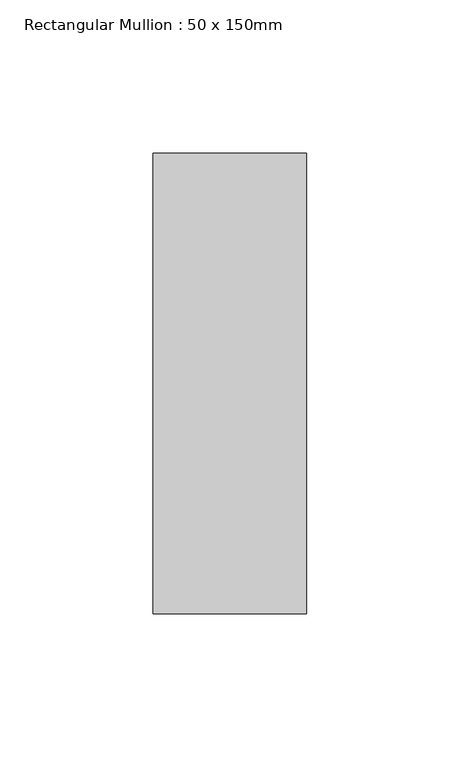
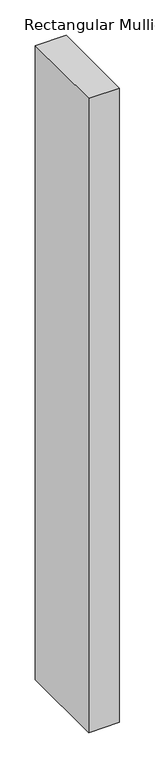
"""IFC4 building model written with IfcOpenShell, lengths in millimetres: member geometry, Rectangular Mullion : 50 x 150mm."""

from ifc_helpers import new_model, si_unit, frame, origin, place, context, project, spatial, polyline, outline, extrude, source, transform, mapped, element, save


def rectangular_mullion_50_x_150mm_71d0ff5f(model_context):
    return source(origin(), model_context, "Body", "SweptSolid", [
        extrude(outline(polyline([(0.0, 75.0), (0.0, -75.0), (-50.0, -75.0), (-50.0, 75.0), (0.0, 75.0)])), frame((0.0, 0.0, -1093.0), z_axis=(0.0, 0.0, 1.0), x_axis=(1.0, 0.0, 0.0)), (0.0, 0.0, 1.0), 1093.0),
    ])


if __name__ == "__main__":
    model = new_model("IFC4")
    model_context = context("Model", 3, world=origin())
    ifc_project = project(units=[si_unit("LENGTHUNIT", "METRE", prefix="MILLI")], contexts=[model_context])
    site = spatial("IfcSite", under=ifc_project)
    building = spatial("IfcBuilding", under=site)
    placement = place(None, origin())
    rectangular_mullion_50_x_150mm_shape = rectangular_mullion_50_x_150mm_71d0ff5f(model_context)
    element("IfcMember", 1, ObjectType="Rectangular Mullion : 50 x 150mm", at=placement, inside=building, context=model_context, shape_type="MappedRepresentation", body=[
        mapped(rectangular_mullion_50_x_150mm_shape, transform((0.0, 0.0, 0.0), x_axis=(1.0, 0.0, 0.0), y_axis=(0.0, 1.0, 0.0), z_axis=(0.0, 0.0, 1.0))),
    ])
    save(model, "model.ifc")

# Revit data of these elements
# Type "Rectangular Mullion : 50 x 150mm"
#   built-in parameter 1007304 = 0.492126 (stored number, unit not read)
#   built-in parameter 1007301 = 0.082021 (stored number, unit not read)
#   built-in parameter 1007300 = 0.082021 (stored number, unit not read)
# Element 1 (IfcMember, "Rectangular Mullion : 50 x 150mm")
#   Materials on its faces: "Aluminium"
# Materials
#   "Aluminium": class "Metal", colour RGB 247 247 247, transparency 0, Description = "Aluminium 6061", Cost = 0
